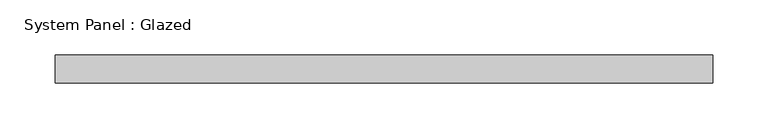
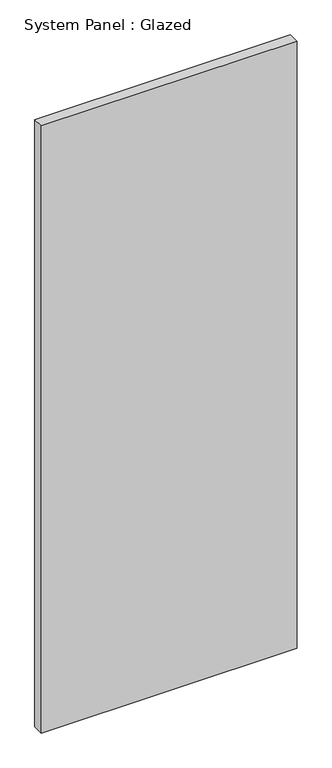
"""IFC4 building model written with IfcOpenShell, lengths in millimetres: plate geometry, System Panel : Glazed."""

from ifc_helpers import new_model, si_unit, origin, origin_with_axes, place, context, project, spatial, polyline, outline, extrude, source, transform, mapped, element, save


def system_panel_glazed_a2afa025(model_context):
    return source(origin(), model_context, "Body", "SweptSolid", [
        extrude(outline(polyline([(298.45, 19.05), (-298.45, 19.05), (-298.45, 44.45), (298.45, 44.45), (298.45, 19.05)])), origin_with_axes(), (0.0, 0.0, 1.0), 1497.1102394),
    ])


if __name__ == "__main__":
    model = new_model("IFC4")
    model_context = context("Model", 3, world=origin())
    ifc_project = project(units=[si_unit("LENGTHUNIT", "METRE", prefix="MILLI")], contexts=[model_context])
    site = spatial("IfcSite", under=ifc_project)
    building = spatial("IfcBuilding", under=site)
    placement = place(None, origin())
    system_panel_glazed_shape = system_panel_glazed_a2afa025(model_context)
    element("IfcPlate", 1, ObjectType="System Panel : Glazed", at=placement, inside=building, context=model_context, shape_type="MappedRepresentation", body=[
        mapped(system_panel_glazed_shape, transform((0.0, 0.0, 0.0), x_axis=(1.0, 0.0, 0.0), y_axis=(0.0, 1.0, 0.0), z_axis=(0.0, 0.0, 1.0))),
    ])
    save(model, "model.ifc")

# Revit data of these elements
# Type "System Panel : Glazed"
#   Construction Type Id = "GSP4R"
#   Analytic Construction = "1/8 in Pilkington single glazing"
#   Visual Light Transmittance = 0.9
#   Solar Heat Gain Coefficient = 0.86
#   Heat Transfer Coefficient (U) = 1.18115 BTU/(h·ft²·°F)
#   Define Thermal Properties by = 1
# Element 1 (IfcPlate, "System Panel : Glazed")
#   Materials on its faces: "Glass"
# Materials
#   "Glass": class "Glass", colour RGB 0 128 192, transparency 0.75, Description = "Soda Lime Glass", Cost = 0
